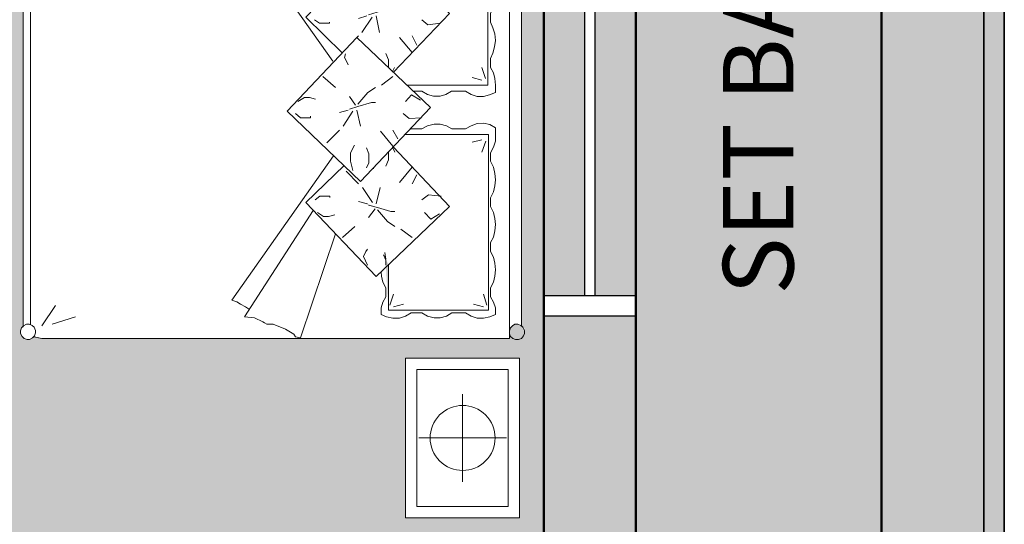
# Model space of a CAD drawing. Units: inches. Extents: x 528 to 2620, y -1066 to 798.
# Tile 14 of 41: x 848 to 944, y 573 to 623. Entities that reach past the tile are written whole.
import ezdxf

# ---------------------------------------------------------------- set-up
doc = ezdxf.new("R2010")
doc.units = ezdxf.units.IN
doc.header["$MEASUREMENT"] = 0
for name, color, linetype, lineweight in [('A-AREA-IDEN', 7, 'Continuous', 18), ('A-FURN', 30, 'Continuous', 18), ('A-GLAZ', 3, 'Continuous', 25), ('A-WALL', 7, 'Continuous', 50), ('A-WALL-PATT', 8, 'Continuous', 13), ('C-PROP', 5, 'Continuous', 35)]:
    doc.layers.add(name, color=color, linetype=linetype, lineweight=lineweight)
doc.styles.get("Standard").update_dxf_attribs({"font": 'arial.ttf'})

# ---------------------------------------------------------------- blocks, each defined once
blk = doc.blocks.new('d-bed-3')
at = {"color": 0, "linetype": 'ByBlock'}
for p, q in [((0, 0), (0, -0.5)), ((0.7, 0), (0, 0)), ((0.7, -0.5), (0.7, 0)), ((0.7817, -0.0054), (0.7857, 0.0078)), ((0.7817, -0.0054), (0.7857, 0.0078)), ((0.7857, 0.0078), (0.7968, 0.0166)), ((0.7857, 0.0078), (0.7968, 0.0166)), ((0.7968, 0.0166), (0.8078, 0.0211)), ((0.7968, 0.0166), (0.8078, 0.0211)), ((0.8078, 0.0211), (0.8209, 0.0211)), ((0.8078, 0.0211), (0.8209, 0.0211)), ((0.8209, 0.0211), (0.8349, 0.0144)), ((0.8209, 0.0211), (0.8349, 0.0144)), ((0.8349, 0.0144), (0.8409, 0.0078)), ((0.8349, 0.0144), (0.8429, 0.0056)), ((0.8389, 0.0078), (2.7305, 0.0078)), ((0.8409, 0.0078), (2.7305, 0.0078)), ((0.8429, 0.0056), (0.848, -0.0077)), ((2.7234, -0.0077), (2.7284, 0.0056)), ((2.7284, 0.0056), (2.7365, 0.0144)), ((2.7305, 0.0078), (2.7365, 0.0144)), ((2.7365, 0.0144), (2.7505, 0.0211)), ((2.7365, 0.0144), (2.7505, 0.0211)), ((2.7505, 0.0211), (2.7636, 0.0211)), ((2.7505, 0.0211), (2.7636, 0.0211)), ((2.7636, 0.0211), (2.7746, 0.0166)), ((2.7636, 0.0211), (2.7746, 0.0166)), ((2.7746, 0.0166), (2.7857, 0.0078)), ((2.7746, 0.0166), (2.7857, 0.0078)), ((2.7857, 0.0078), (2.7897, -0.0054)), ((2.7857, 0.0078), (2.7897, -0.0054)), ((2.8714, -0.5), (2.8714, 0)), ((2.8714, 0), (3.5714, 0)), ((3.5714, 0), (3.5714, -0.5)), ((0.7817, -0.0187), (0.7817, -0.0054)), ((0.7817, -0.0187), (0.7817, -0.0054)), ((0.7857, -0.0297), (0.7817, -0.0187)), ((0.7857, -0.0297), (0.7817, -0.0187)), ((0.7857, -2.0939), (0.7857, -0.0297)), ((0.7948, -0.0408), (0.7857, -0.0297)), ((0.7857, -0.032), (0.7857, -2.0939)), ((0.8058, -0.0452), (0.7948, -0.0408)), ((0.8319, -0.0408), (0.8188, -0.0452)), ((0.8409, -0.032), (0.8319, -0.0408)), ((0.848, -0.0209), (0.8409, -0.032)), ((0.848, -0.0077), (0.848, -0.0209)), ((2.7234, -0.0209), (2.7234, -0.0077)), ((2.7305, -0.032), (2.7234, -0.0209)), ((2.7395, -0.0408), (2.7305, -0.032)), ((2.7525, -0.0452), (2.7395, -0.0408)), ((2.7766, -0.0408), (2.7656, -0.0452)), ((2.7766, -0.0408), (2.7656, -0.0452)), ((2.7857, -0.0297), (2.7766, -0.0408)), ((2.7857, -0.0297), (2.7766, -0.0408)), ((2.7897, -0.0187), (2.7857, -0.0297)), ((2.7897, -0.0187), (2.7857, -0.0297)), ((2.7897, -0.0054), (2.7897, -0.0187)), ((2.7897, -0.0054), (2.7897, -0.0187)), ((0.05, -0.05), (0.05, -0.45)), ((0.65, -0.05), (0.05, -0.05)), ((0.35, -0.0576), (0.35, -0.4424)), ((0.65, -0.45), (0.65, -0.05)), ((0.8188, -0.0452), (0.8058, -0.0452)), ((2.7525, -0.0452), (0.8188, -0.0452)), ((2.7656, -0.0452), (2.7525, -0.0452)), ((2.7656, -0.0452), (2.7857, -0.0452)), ((2.7857, -0.0452), (2.7656, -0.0452)), ((2.7857, -2.0939), (2.7857, -0.0452)), ((2.9214, -0.45), (2.9214, -0.05)), ((2.9214, -0.05), (3.5214, -0.05)), ((3.2214, -0.0576), (3.2214, -0.4424)), ((3.5214, -0.05), (3.5214, -0.45)), ((0.8781, -0.1325), (0.8911, -0.1059)), ((0.8911, -0.1059), (0.9182, -0.1082)), ((0.9182, -0.1082), (0.9443, -0.1148)), ((0.9443, -0.1148), (0.9684, -0.128)), ((0.9684, -0.128), (1.0056, -0.128)), ((1.0056, -0.128), (1.0317, -0.117)), ((1.0317, -0.117), (1.0588, -0.1082)), ((1.0588, -0.1082), (1.0849, -0.1059)), ((1.0849, -0.1059), (1.113, -0.1104)), ((1.113, -0.1104), (1.1401, -0.117)), ((1.1401, -0.117), (1.1662, -0.128)), ((1.1662, -0.128), (1.2034, -0.128)), ((1.2034, -0.128), (1.2295, -0.117)), ((1.2295, -0.117), (1.2566, -0.1082)), ((1.2566, -0.1082), (1.2827, -0.1059)), ((1.2827, -0.1059), (1.3108, -0.1104)), ((1.3108, -0.1104), (1.3379, -0.117)), ((1.3379, -0.117), (1.362, -0.128)), ((1.362, -0.128), (1.4012, -0.128)), ((1.4012, -0.128), (1.4253, -0.117)), ((1.4253, -0.117), (1.4514, -0.1082)), ((1.4514, -0.1082), (1.4805, -0.1059)), ((1.4805, -0.1059), (1.5086, -0.1104)), ((1.5086, -0.1104), (1.5357, -0.117)), ((1.5357, -0.117), (1.5598, -0.128)), ((1.5598, -0.128), (1.5989, -0.128)), ((1.5989, -0.128), (1.623, -0.1148)), ((1.623, -0.1148), (1.6471, -0.1082)), ((1.6471, -0.1082), (1.6763, -0.1059)), ((1.6763, -0.1059), (1.7084, -0.1059)), ((1.7084, -0.1059), (1.7194, -0.1325)), ((1.8489, -0.1302), (1.863, -0.1059)), ((1.863, -0.1059), (1.8951, -0.1059)), ((1.8951, -0.1059), (1.9222, -0.1059)), ((1.9222, -0.1059), (1.9483, -0.1148)), ((1.9483, -0.1148), (1.9724, -0.128)), ((1.9724, -0.128), (2.0096, -0.128)), ((2.0096, -0.128), (2.0357, -0.1148)), ((2.0357, -0.1148), (2.0628, -0.1082)), ((2.0628, -0.1082), (2.0909, -0.1059)), ((2.0909, -0.1059), (2.117, -0.1082)), ((2.117, -0.1082), (2.1441, -0.1148)), ((2.1441, -0.1148), (2.1702, -0.128)), ((2.1702, -0.128), (2.2074, -0.128)), ((2.2074, -0.128), (2.2335, -0.1148)), ((2.2335, -0.1148), (2.2606, -0.1082)), ((2.2606, -0.1082), (2.2867, -0.1059)), ((2.2867, -0.1059), (2.3148, -0.1082)), ((2.3148, -0.1082), (2.3419, -0.1148)), ((2.3419, -0.1148), (2.366, -0.128)), ((2.366, -0.128), (2.4052, -0.128)), ((2.4052, -0.128), (2.4293, -0.1148)), ((2.4293, -0.1148), (2.4554, -0.1082)), ((2.4554, -0.1082), (2.4845, -0.1059)), ((2.4845, -0.1059), (2.5126, -0.1082)), ((2.5126, -0.1082), (2.5397, -0.1148)), ((2.5397, -0.1148), (2.5638, -0.128)), ((2.5638, -0.128), (2.6029, -0.128)), ((2.6029, -0.128), (2.627, -0.1148)), ((2.627, -0.1148), (2.6511, -0.1059)), ((2.6511, -0.1059), (2.6803, -0.1059)), ((2.6803, -0.1059), (2.6913, -0.1302)), ((0.8721, -0.159), (0.8781, -0.1325)), ((0.8741, -0.1866), (0.8721, -0.159)), ((0.9072, -0.5753), (0.9072, -0.1391)), ((0.9072, -0.1391), (1.6763, -0.1391)), ((0.9223, -0.1612), (0.9333, -0.2042)), ((0.9293, -0.1435), (0.9775, -0.1612)), ((1.6471, -0.1501), (1.5989, -0.1656)), ((1.6542, -0.1656), (1.6431, -0.2087)), ((1.6763, -0.1391), (1.6763, -0.4936)), ((1.7194, -0.1325), (1.7265, -0.159)), ((1.7265, -0.159), (1.7265, -0.1866)), ((1.8429, -0.159), (1.8489, -0.1302)), ((1.8449, -0.1866), (1.8429, -0.159)), ((2.6622, -0.1369), (1.8931, -0.1369)), ((1.8931, -0.1369), (1.8931, -0.5046)), ((1.9152, -0.1656), (1.9263, -0.2087)), ((1.9222, -0.1479), (1.9704, -0.1656)), ((2.6401, -0.1435), (2.5919, -0.159)), ((2.6471, -0.159), (2.6361, -0.202)), ((2.6622, -0.5753), (2.6622, -0.1369)), ((2.6913, -0.1302), (2.6973, -0.159)), ((2.6973, -0.159), (2.6973, -0.1866)), ((0.8831, -0.2131), (0.8741, -0.1866)), ((0.8962, -0.2374), (0.8831, -0.2131)), ((1.7174, -0.2131), (1.7024, -0.2374)), ((1.7265, -0.1866), (1.7174, -0.2131)), ((1.854, -0.2131), (1.8449, -0.1866)), ((1.867, -0.2374), (1.854, -0.2131)), ((2.6883, -0.2131), (2.6732, -0.2374)), ((2.6973, -0.1866), (2.6883, -0.2131)), ((0.1576, -0.25), (0.5424, -0.25)), ((0.8962, -0.2992), (0.8962, -0.2374)), ((1.7024, -0.2374), (1.7024, -0.2992)), ((1.867, -0.297), (1.867, -0.2374)), ((2.6732, -0.2374), (2.6732, -0.297)), ((3.4138, -0.25), (3.029, -0.25)), ((0.8831, -0.3235), (0.8962, -0.2992)), ((1.7024, -0.2992), (1.7174, -0.3235)), ((1.854, -0.3213), (1.867, -0.297)), ((2.6732, -0.297), (2.6883, -0.3213)), ((0.8761, -0.3489), (0.8831, -0.3235)), ((1.0538, -0.6294), (1.362, -0.3081)), ((1.362, -0.3081), (1.619, -0.5532)), ((1.7174, -0.3235), (1.7244, -0.3489)), ((1.8469, -0.3489), (1.854, -0.3213)), ((2.2074, -0.3081), (1.9483, -0.5532)), ((2.1632, -0.3445), (2.1572, -0.3997)), ((2.5146, -0.6294), (2.2074, -0.3081)), ((2.6883, -0.3213), (2.6953, -0.3489)), ((0.8761, -0.3776), (0.8761, -0.3489)), ((0.8831, -0.4041), (0.8761, -0.3776)), ((1.3289, -0.3511), (1.3068, -0.3909)), ((1.4052, -0.3467), (1.4122, -0.4019)), ((1.7244, -0.3776), (1.7174, -0.4041)), ((1.7244, -0.3489), (1.7244, -0.3776)), ((1.8469, -0.3754), (1.8469, -0.3489)), ((1.854, -0.4041), (1.8469, -0.3754)), ((2.2405, -0.3511), (2.2626, -0.3887)), ((2.6953, -0.3754), (2.6883, -0.4041)), ((2.6953, -0.3489), (2.6953, -0.3754)), ((0.8962, -0.4284), (0.8831, -0.4041)), ((0.8962, -0.4781), (0.8962, -0.4284)), ((1.3068, -0.3909), (1.3349, -0.4174)), ((1.4122, -0.4019), (1.3901, -0.4284)), ((1.4674, -0.7134), (1.7746, -0.3909)), ((1.7174, -0.4041), (1.7024, -0.4284)), ((1.7024, -0.4284), (1.7024, -0.4649)), ((1.7746, -0.3909), (2.0979, -0.6979)), ((1.8188, -0.4306), (1.8228, -0.4848)), ((1.867, -0.4284), (1.854, -0.4041)), ((1.867, -0.4781), (1.867, -0.4284)), ((2.1572, -0.3997), (2.1793, -0.4284)), ((2.2626, -0.3887), (2.2335, -0.4174)), ((2.6883, -0.4041), (2.6732, -0.4284)), ((2.6732, -0.4284), (2.6732, -0.4759)), ((0.05, -0.45), (0.65, -0.45)), ((1.2255, -0.4715), (1.2626, -0.5223)), ((1.5006, -0.4505), (1.4604, -0.4715)), ((1.5327, -0.4715), (1.4674, -0.5267)), ((1.7415, -0.4351), (1.7194, -0.4737)), ((1.7194, -0.4737), (1.7485, -0.5002)), ((2.0357, -0.4715), (2.102, -0.5267)), ((2.0688, -0.4505), (2.109, -0.4715)), ((2.3439, -0.4715), (2.3068, -0.5201)), ((3.5214, -0.45), (2.9214, -0.45)), ((0, -0.5), (0.7, -0.5)), ((0.8741, -0.5289), (0.8831, -0.5024)), ((0.8831, -0.5024), (0.8962, -0.4781)), ((0.9223, -0.5532), (0.9333, -0.5113)), ((1.8228, -0.4848), (1.8008, -0.5113)), ((2.6471, -0.5532), (2.6361, -0.5091)), ((2.6732, -0.4759), (2.6883, -0.5002)), ((2.6883, -0.5002), (2.6973, -0.5267)), ((3.5714, -0.5), (2.8714, -0.5)), ((0.8721, -0.5576), (0.8741, -0.5289)), ((0.8781, -0.5841), (0.8721, -0.5576)), ((0.9293, -0.5709), (0.9775, -0.5532)), ((1.2957, -0.5819), (1.2737, -0.5488)), ((1.3399, -0.5643), (1.3399, -0.5488)), ((1.5989, -0.5488), (1.614, -0.5554)), ((1.6381, -0.5554), (1.6763, -0.6051)), ((1.9112, -0.5333), (1.874, -0.5554)), ((1.9443, -0.5554), (1.8781, -0.6096)), ((1.9704, -0.5466), (1.9503, -0.5554)), ((2.2295, -0.5643), (2.2295, -0.5466)), ((2.2736, -0.5797), (2.2957, -0.5466)), ((2.6401, -0.5687), (2.5919, -0.5532)), ((2.6973, -0.5554), (2.6913, -0.5841)), ((2.6973, -0.5267), (2.6973, -0.5554)), ((0.8911, -0.6096), (0.8781, -0.5841)), ((1.109, -0.5753), (0.9072, -0.5753)), ((0.9443, -0.6007), (0.9182, -0.6073)), ((0.9684, -0.5886), (0.9443, -0.6007)), ((1.0056, -0.5886), (0.9684, -0.5886)), ((1.0317, -0.5996), (1.0056, -0.5886)), ((1.0588, -0.6073), (1.0317, -0.5996)), ((1.105, -0.5864), (1.1271, -0.5864)), ((1.1271, -0.5864), (1.1482, -0.5974)), ((1.1482, -0.5974), (1.1311, -0.5864)), ((1.1311, -0.5864), (1.1592, -0.593)), ((1.3459, -0.625), (1.2957, -0.5819)), ((1.357, -0.625), (1.3399, -0.5643)), ((1.5658, -0.5753), (1.5377, -0.5864)), ((1.5969, -0.5753), (1.5658, -0.5753)), ((1.9684, -0.5753), (2.0036, -0.5753)), ((2.0036, -0.5753), (2.0317, -0.5864)), ((2.2124, -0.6228), (2.2295, -0.5643)), ((2.2224, -0.6228), (2.2736, -0.5797)), ((2.4383, -0.5864), (2.4092, -0.5908)), ((2.4423, -0.5864), (2.4202, -0.5974)), ((2.4202, -0.5974), (2.4383, -0.5864)), ((2.4644, -0.5864), (2.4423, -0.5864)), ((2.4604, -0.5753), (2.6622, -0.5753)), ((2.5397, -0.5996), (2.5126, -0.6051)), ((2.5638, -0.5864), (2.5397, -0.5996)), ((2.6029, -0.5864), (2.5638, -0.5864)), ((2.627, -0.5996), (2.6029, -0.5864)), ((2.6511, -0.6073), (2.627, -0.5996)), ((2.6913, -0.5841), (2.6803, -0.6073)), ((0.9182, -0.6073), (0.8911, -0.6096)), ((1.3791, -0.9365), (1.0538, -0.6294)), ((1.0759, -0.6096), (1.0588, -0.6073)), ((1.3138, -0.6626), (1.351, -0.6361)), ((1.368, -0.6626), (1.357, -0.625)), ((1.3731, -0.6294), (1.4453, -0.614)), ((1.3791, -0.6471), (1.4453, -0.6913)), ((1.7084, -0.6648), (1.6873, -0.6316)), ((1.7526, -0.6493), (1.7526, -0.6316)), ((2.0387, -0.6427), (2.0427, -0.6405)), ((2.1963, -0.6294), (2.124, -0.6118)), ((2.1903, -0.6449), (2.124, -0.6891)), ((2.1903, -0.9365), (2.5146, -0.6294)), ((2.2013, -0.6626), (2.2124, -0.6228)), ((2.2556, -0.6626), (2.2184, -0.6338)), ((2.5126, -0.6051), (2.4955, -0.6073)), ((2.6803, -0.6073), (2.6511, -0.6073)), ((1.105, -0.6692), (1.1421, -0.6846)), ((1.1421, -0.6846), (1.1642, -0.6736)), ((1.1642, -0.6736), (1.1753, -0.6692)), ((1.3731, -0.6692), (1.3841, -0.7067)), ((1.7596, -0.7089), (1.7084, -0.6648)), ((1.7706, -0.7089), (1.7526, -0.6493)), ((1.9765, -0.6604), (1.9503, -0.6714)), ((2.0166, -0.6604), (1.9765, -0.6604)), ((2.0387, -0.6714), (2.0166, -0.6604)), ((2.1963, -0.667), (2.1853, -0.7067)), ((2.4052, -0.6736), (2.3941, -0.667)), ((2.4272, -0.6846), (2.4052, -0.6736)), ((2.4644, -0.667), (2.4272, -0.6846)), ((1.2255, -0.7785), (1.2737, -0.7244)), ((1.4674, -0.7134), (1.4604, -0.7067)), ((1.7897, -1.0193), (1.4674, -0.7134)), ((1.7265, -0.7454), (1.7636, -0.72)), ((1.7817, -0.7454), (1.7706, -0.7089)), ((1.7857, -0.7134), (1.856, -0.6979)), ((2.0979, -0.6979), (1.7897, -1.0193)), ((1.7897, -0.731), (1.856, -0.7741)), ((1.9724, -0.741), (1.9393, -0.7244)), ((2.0497, -0.731), (2.0096, -0.741)), ((2.0538, -0.7609), (2.109, -0.7067)), ((2.3439, -0.7763), (2.2957, -0.7222)), ((1.3791, -0.9365), (1.5357, -0.7763)), ((1.5548, -0.7675), (1.5397, -0.7631)), ((1.5548, -0.7675), (1.5769, -0.7564)), ((1.5769, -0.7564), (1.5879, -0.752)), ((1.7857, -0.752), (1.7967, -0.7896)), ((2.0096, -0.741), (1.9724, -0.741)), ((2.1903, -0.9365), (2.0277, -0.7697)), ((0.7857, -0.9607), (1.2295, -0.8072)), ((0.9504, -1.2611), (1.5708, -0.8183)), ((1.3178, -0.8382), (1.3239, -0.8117)), ((1.6381, -0.8625), (1.6873, -0.8072)), ((1.9283, -0.8448), (1.874, -0.7896)), ((2.618, -1.2611), (1.9855, -0.8161)), ((2.2515, -0.8382), (2.2445, -0.8094)), ((2.7827, -0.9607), (2.3278, -0.8072)), ((1.3178, -0.8602), (1.3178, -0.8382)), ((1.3349, -0.8879), (1.3178, -0.8602)), ((1.4052, -0.8337), (1.4012, -0.8337)), ((1.4052, -0.8768), (1.4052, -0.8337)), ((2.1632, -0.8757), (2.1632, -0.8315)), ((2.1632, -0.8315), (2.1682, -0.8315)), ((2.2335, -0.8856), (2.2515, -0.8602)), ((2.2515, -0.8602), (2.2515, -0.8382)), ((0.8781, -1.2059), (1.3349, -0.9055)), ((1.3901, -0.8989), (1.4052, -0.8768)), ((1.7305, -0.921), (1.7375, -0.8945)), ((2.1793, -0.8967), (2.1632, -0.8757)), ((2.6913, -1.2059), (2.2254, -0.9055)), ((1.7305, -0.9431), (1.7305, -0.921)), ((1.7485, -0.9718), (1.7305, -0.9431)), ((1.8188, -0.9166), (1.8118, -0.9166)), ((1.8188, -0.9607), (1.8188, -0.9166)), ((0.8128, -1.0115), (0.7857, -0.9607)), ((1.8008, -0.9828), (1.8188, -0.9607)), ((2.7676, -0.9895), (2.7455, -1.0259)), ((2.7786, -0.9828), (2.7676, -0.9895)), ((2.7827, -0.9607), (2.7786, -0.9828)), ((0.8128, -1.0325), (0.8128, -1.0115)), ((0.8239, -1.0414), (0.8128, -1.0325)), ((2.7455, -1.0259), (2.7234, -1.0811)), ((0.8299, -1.0635), (0.8239, -1.0414)), ((0.8349, -1.0745), (0.8299, -1.0635)), ((0.845, -1.1032), (0.8349, -1.0745)), ((0.852, -1.1187), (0.845, -1.1032)), ((0.852, -1.1363), (0.852, -1.1187)), ((2.7174, -1.1187), (2.7124, -1.1253)), ((2.7234, -1.1076), (2.7174, -1.1187)), ((2.7234, -1.0811), (2.7234, -1.1076)), ((0.863, -1.1617), (0.852, -1.1363)), ((0.867, -1.1905), (0.863, -1.1617)), ((2.6953, -1.1617), (2.6913, -1.2059)), ((2.7124, -1.1253), (2.6953, -1.1617)), ((0.8741, -1.1949), (0.867, -1.1905)), ((0.8781, -1.2059), (0.8741, -1.1949)), ((0.9223, -1.2015), (0.9112, -1.1838)), ((0.9293, -1.2059), (0.9223, -1.2015)), ((0.9403, -1.2236), (0.9293, -1.2059)), ((2.6471, -1.2015), (2.6361, -1.2236)), ((2.6582, -1.1838), (2.6471, -1.2015)), ((0.9443, -1.2391), (0.9403, -1.2236)), ((0.9504, -1.2611), (0.9443, -1.2391)), ((2.625, -1.2391), (2.618, -1.2611)), ((2.6361, -1.2236), (2.625, -1.2391)), ((0.8741, -2.0673), (0.9464, -1.9691)), ((2.7234, -2.0497), (2.6913, -1.947)), ((0.8851, -2.1005), (0.9795, -2.0342)), ((2.7305, -2.0939), (2.6421, -2.0342)), ((0.7888, -2.1317), (0.7857, -2.0939)), ((0.7857, -2.0939), (0.7887, -2.1303)), ((2.7857, -2.0939), (2.7783, -2.1299)), ((2.7786, -2.1281), (2.7857, -2.0939)), ((0.7797, -2.148), (0.7857, -2.1347)), ((0.7797, -2.148), (0.7857, -2.1347)), ((0.7797, -2.159), (0.7797, -2.148)), ((0.7797, -2.148), (0.7797, -2.159)), ((0.7857, -2.1347), (0.7948, -2.1259)), ((0.7857, -2.1347), (0.7888, -2.1317)), ((0.7948, -2.1259), (0.8078, -2.1215)), ((0.8078, -2.1215), (0.8188, -2.1215)), ((0.8188, -2.1215), (0.8319, -2.1281)), ((0.8319, -2.1281), (0.8409, -2.1369)), ((0.8409, -2.1369), (0.845, -2.1502)), ((2.7264, -2.1436), (0.845, -2.1436)), ((0.845, -2.1502), (0.845, -2.1612)), ((2.7284, -2.1369), (2.7234, -2.1502)), ((2.7234, -2.1502), (2.7234, -2.1612)), ((2.7365, -2.1281), (2.7284, -2.1369)), ((2.7505, -2.1215), (2.7365, -2.1281)), ((2.7616, -2.1215), (2.7505, -2.1215)), ((2.7746, -2.1259), (2.7616, -2.1215)), ((2.7827, -2.1347), (2.7746, -2.1259)), ((2.7783, -2.1299), (2.7827, -2.1347)), ((2.7827, -2.1347), (2.7897, -2.148)), ((2.7897, -2.148), (2.7827, -2.1347)), ((2.7897, -2.148), (2.7897, -2.159)), ((2.7897, -2.159), (2.7897, -2.148)), ((0.7837, -2.1723), (0.7797, -2.159)), ((0.7837, -2.1723), (0.7797, -2.159)), ((0.7927, -2.1811), (0.7837, -2.1723)), ((0.7927, -2.1811), (0.7837, -2.1723)), ((0.8058, -2.1877), (0.7927, -2.1811)), ((0.8058, -2.1877), (0.7927, -2.1811)), ((0.8168, -2.1877), (0.8058, -2.1877)), ((0.8168, -2.1877), (0.8058, -2.1877)), ((0.8299, -2.1833), (0.8168, -2.1877)), ((0.8299, -2.1833), (0.8168, -2.1877)), ((0.8389, -2.1745), (0.8299, -2.1833)), ((0.8367, -2.1767), (0.8299, -2.1833)), ((2.7327, -2.1767), (0.8367, -2.1767)), ((0.845, -2.1612), (0.8389, -2.1745)), ((0.8389, -2.1767), (2.7305, -2.1767)), ((2.7234, -2.1612), (2.7305, -2.1745)), ((2.7305, -2.1745), (2.7395, -2.1833)), ((2.7395, -2.1833), (2.7327, -2.1767)), ((2.7525, -2.1877), (2.7395, -2.1833)), ((2.7395, -2.1833), (2.7525, -2.1877)), ((2.7636, -2.1877), (2.7525, -2.1877)), ((2.7525, -2.1877), (2.7636, -2.1877)), ((2.7766, -2.1811), (2.7636, -2.1877)), ((2.7636, -2.1877), (2.7766, -2.1811)), ((2.7857, -2.1723), (2.7766, -2.1811)), ((2.7766, -2.1811), (2.7857, -2.1723)), ((2.7897, -2.159), (2.7857, -2.1723)), ((2.7857, -2.1723), (2.7897, -2.159))]:
    blk.add_line(p, q, dxfattribs=at)
blk.add_ellipse((0.35, -0.25), major_axis=(-0.1007, 0.1007), ratio=1, dxfattribs=at)
at = {"color": 0, "linetype": 'ByBlock', "extrusion": (0, 0, -1)}
blk.add_ellipse((3.2214, -0.25), major_axis=(0.1007, 0.1007), ratio=1, dxfattribs=at)
blk = doc.blocks.new('WIN-1200')
for p, q in [((677.559, 718.922), (725.559, 718.922)), ((677.559, 709.922), (677.559, 718.922)), ((679.559, 709.922), (679.559, 718.922)), ((723.559, 718.922), (723.559, 709.922)), ((725.559, 718.922), (725.559, 709.922)), ((679.559, 714.922), (723.559, 714.922)), ((679.559, 713.922), (723.559, 713.922)), ((725.559, 709.922), (677.559, 709.922))]:
    blk.add_line(p, q)

msp = doc.modelspace()

# ---------------------------------------------------------------- hatches: boundary and pattern name
at = {"layer": 'A-WALL-PATT', "transparency": 33554687}
h = msp.add_hatch(color=256, dxfattribs=at)
h.dxf.hatch_style = 1
h.paths.add_polyline_path([(944.059, 753.922), (584.059, 753.922), (584.059, 208.922), (608.059, 208.922), (608.059, 210.922), (586.059, 210.922), (586.059, 751.922), (942.059, 751.922), (942.059, 210.922), (728.059, 210.922), (728.059, 208.922), (944.059, 208.922)])
h = msp.add_hatch(color=256, dxfattribs=at)
h.dxf.hatch_style = 1
h.paths.add_polyline_path([(942.059, 751.922), (586.059, 751.922), (586.059, 210.922), (608.059, 210.922), (608.059, 220.922), (596.059, 220.922), (596.059, 741.922), (932.059, 741.922), (932.059, 220.922), (770.059, 220.922), (728.059, 220.922), (728.059, 210.922), (942.059, 210.922)])
at = {"layer": 'A-WALL-PATT', "transparency": 33554475}
h = msp.add_hatch(color=256, dxfattribs=at)
h.dxf.hatch_style = 1
h.paths.add_polyline_path([(620.059, 718.922), (908.059, 718.922), (908.059, 268.922), (770.059, 268.922), (770.059, 220.922), (932.059, 220.922), (932.059, 741.922), (596.059, 741.922), (596.059, 391.422), (620.059, 391.422)])
at = {"layer": 'A-WALL-PATT', "transparency": 33554687}
h = msp.add_hatch(color=256, dxfattribs=at)
h.dxf.hatch_style = 1
h.paths.add_polyline_path([(861.059, 273.922), (817.059, 273.922), (817.059, 272.922), (861.059, 272.922)])
h.paths.add_polyline_path([(817.059, 277.922), (815.059, 277.922), (815.059, 268.922), (817.059, 268.922)])
h.paths.add_polyline_path([(908.059, 397.922), (899.059, 397.922), (899.059, 395.922), (908.059, 395.922)])
h.paths.add_polyline_path([(908.059, 443.922), (899.059, 443.922), (899.059, 441.922), (908.059, 441.922)])
h.paths.add_polyline_path([(904.059, 441.922), (903.059, 441.922), (903.059, 397.922), (904.059, 397.922)])
h.paths.add_polyline_path([(625.059, 561.422), (624.059, 561.422), (624.059, 537.422), (625.059, 537.422)])
h.paths.add_polyline_path([(648.747, 334.444), (720.045, 334.444), (720.045, 344.998), (648.747, 344.998)], flags=9)
h.paths.add_polyline_path([(819.733, 323.153), (880.328, 323.153), (880.328, 333.708), (819.733, 333.708)], flags=9)
h.paths.add_polyline_path([(779.898, 680.607), (821.764, 680.607), (821.764, 691.169), (779.898, 691.169)], flags=9)
h.paths.add_polyline_path([(779.876, 692.362), (817.138, 692.362), (817.138, 703.058), (779.876, 703.058)], flags=9)
h.paths.add_polyline_path([(799.994, 453.884), (860.589, 453.884), (860.589, 464.439), (799.994, 464.439)], flags=9)
h.paths.add_polyline_path([(650.866, 539.397), (708.781, 539.397), (708.781, 549.952), (650.866, 549.952)], flags=9)
h.paths.add_polyline_path([(788.504, 612.01), (849.099, 612.01), (849.099, 622.565), (788.504, 622.565)], flags=9)
h.paths.add_polyline_path([(639.539, 648.31), (700.134, 648.31), (700.134, 658.865), (639.539, 658.865)], flags=9)
h.paths.add_polyline_path([(648.913, 346.09), (747.706, 346.09), (747.706, 356.778), (648.913, 356.778)], flags=9)
h.paths.add_polyline_path([(676.857, 450.66), (746.735, 450.66), (746.735, 461.355), (676.857, 461.355)], flags=9)
h.paths.add_polyline_path([(819.711, 334.947), (865.526, 334.947), (865.526, 345.636), (819.711, 345.636)], flags=9)
h.paths.add_polyline_path([(806.298, 467.745), (874.047, 467.745), (874.047, 478.441), (806.298, 478.441)], flags=9)
h.paths.add_polyline_path([(653.235, 552.284), (690.497, 552.284), (690.497, 562.979), (653.235, 562.979)], flags=9)
h.paths.add_polyline_path([(789.903, 623.407), (843.208, 623.407), (843.208, 634.103), (789.903, 634.103)], flags=9)
h.paths.add_polyline_path([(639.773, 662.103), (693.077, 662.103), (693.077, 672.798), (639.773, 672.798)], flags=9)
h.paths.add_polyline_path([(801.587, 242.914), (846.334, 242.914), (846.334, 253.603), (801.587, 253.603)], flags=9)
h.paths.add_polyline_path([(925.362, 593.982), (925.362, 674.057), (914.673, 674.057), (914.673, 593.982)], flags=9)
h.paths.add_polyline_path([(612.559, 593.982), (612.559, 674.057), (601.871, 674.057), (601.871, 593.982)], flags=9)
h.paths.add_polyline_path([(723.31, 726.564), (803.385, 726.564), (803.385, 737.252), (723.31, 737.252)], flags=9)
at = {"layer": 'A-WALL-PATT', "transparency": 33554521}
h = msp.add_hatch(color=256, dxfattribs=at)
h.dxf.hatch_style = 1
h.paths.add_polyline_path([(629.059, 709.922), (677.559, 709.922), (677.559, 718.922), (620.059, 718.922), (620.059, 667.922), (629.059, 667.922)])
h.paths.add_polyline_path([(790.559, 718.922), (725.559, 718.922), (725.559, 709.922), (774.059, 709.922), (774.059, 577.922), (768.481, 577.922), (768.559, 573.422), (774.059, 573.422), (774.059, 567.422), (778.559, 567.422), (778.559, 669.422), (831.059, 669.422), (831.059, 675.922), (826.559, 675.922), (826.559, 673.922), (778.559, 673.922), (778.559, 709.922), (790.559, 709.922)])
h.paths.add_polyline_path([(908.059, 718.922), (879.059, 718.922), (879.059, 709.922), (899.059, 709.922), (899.059, 641.672), (908.059, 641.672)])
h.paths.add_polyline_path([(629.059, 619.922), (620.059, 619.922), (620.059, 561.422), (629.059, 561.422), (629.059, 573.422), (724.059, 573.422), (724.059, 569.422), (728.559, 569.422), (728.559, 577.922), (629.059, 577.922)])
h.paths.add_polyline_path([(779.059, 391.422), (779.059, 400.422), (770.059, 400.422), (764.059, 400.422), (764.059, 397.422), (764.059, 391.422), (770.059, 391.422), (770.059, 268.922), (815.059, 268.922), (815.059, 277.922), (779.059, 277.922), (779.059, 359.767)])
h.paths.add_polyline_path([(908.059, 395.922), (899.059, 395.922), (851.059, 395.922), (851.059, 391.422), (899.059, 391.422), (899.059, 277.922), (863.059, 277.922), (863.059, 268.922), (908.059, 268.922)])
h.paths.add_polyline_path([(908.059, 593.672), (899.059, 593.672), (899.059, 525.422), (778.559, 525.422), (778.559, 527.172), (774.059, 527.172), (774.059, 520.922), (899.059, 520.922), (899.059, 443.922), (908.059, 443.922)])
h.paths.add_polyline_path([(629.059, 520.922), (728.559, 520.922), (728.559, 545.422), (724.059, 545.422), (724.059, 525.422), (629.059, 525.422), (629.059, 537.422), (620.059, 537.422), (620.059, 484.672), (629.059, 484.672)])
h.paths.add_polyline_path([(629.059, 436.672), (620.059, 436.672), (620.059, 391.422), (648.559, 391.422), (648.559, 400.422), (629.059, 400.422)])
h.paths.add_polyline_path([(716.059, 397.422), (716.059, 400.422), (696.559, 400.422), (696.559, 391.422), (716.059, 391.422)])
at = {"layer": 'A-WALL-PATT', "transparency": 33554681}
h = msp.add_hatch(color=256, dxfattribs=at)
h.dxf.hatch_style = 1
h.paths.add_polyline_path([(629.059, 665.922), (625.059, 665.922), (625.059, 621.922), (629.059, 621.922)])
h.paths.add_polyline_path([(624.059, 665.922), (620.059, 665.922), (620.059, 621.922), (624.059, 621.922)])
h.paths.add_polyline_path([(723.559, 713.922), (679.559, 713.922), (679.559, 709.922), (723.559, 709.922)])
h.paths.add_polyline_path([(723.559, 718.922), (679.559, 718.922), (679.559, 714.922), (723.559, 714.922)])
h.paths.add_polyline_path([(814.559, 713.922), (790.559, 713.922), (790.559, 709.922), (814.559, 709.922)])
h.paths.add_polyline_path([(814.559, 718.922), (790.559, 718.922), (790.559, 714.922), (814.559, 714.922)])
h.paths.add_polyline_path([(877.059, 713.922), (833.059, 713.922), (833.059, 709.922), (877.059, 709.922)])
h.paths.add_polyline_path([(877.059, 718.922), (833.059, 718.922), (833.059, 714.922), (877.059, 714.922)])
h.paths.add_polyline_path([(908.059, 639.672), (904.059, 639.672), (904.059, 595.672), (908.059, 595.672)])
h.paths.add_polyline_path([(903.059, 639.672), (899.059, 639.672), (899.059, 595.672), (903.059, 595.672)])
h.paths.add_polyline_path([(908.059, 441.922), (904.059, 441.922), (904.059, 397.922), (908.059, 397.922)])
h.paths.add_polyline_path([(903.059, 441.922), (899.059, 441.922), (899.059, 397.922), (903.059, 397.922)])
h.paths.add_polyline_path([(861.059, 272.922), (817.059, 272.922), (817.059, 268.922), (861.059, 268.922)])
h.paths.add_polyline_path([(861.059, 277.922), (817.059, 277.922), (817.059, 273.922), (861.059, 273.922)])
h.paths.add_polyline_path([(694.559, 395.422), (650.559, 395.422), (650.559, 391.422), (694.559, 391.422)])
h.paths.add_polyline_path([(694.559, 400.422), (650.559, 400.422), (650.559, 396.422), (694.559, 396.422)])
h.paths.add_polyline_path([(629.059, 482.672), (625.059, 482.672), (625.059, 438.672), (629.059, 438.672)])
h.paths.add_polyline_path([(624.059, 482.672), (620.059, 482.672), (620.059, 438.672), (624.059, 438.672)])
h.paths.add_polyline_path([(629.059, 561.422), (625.059, 561.422), (625.059, 537.422), (629.059, 537.422)])
h.paths.add_polyline_path([(624.059, 561.422), (620.059, 561.422), (620.059, 537.422), (624.059, 537.422)])
at = {"layer": 'A-WALL-PATT', "transparency": 33554590}
h = msp.add_hatch(color=256, dxfattribs=at)
h.dxf.hatch_style = 1
h.paths.add_polyline_path([(774.059, 709.922), (629.059, 709.922), (629.059, 577.922), (728.559, 577.922), (728.559, 579.422), (728.559, 619.422), (730.309, 619.422), (730.309, 619.384, -0.401453), (768.559, 579.422), (768.559, 577.922), (774.059, 577.922)])
h.paths.add_polyline_path([(723.896, 686.058), (723.968, 686.064), (723.828, 686.128)], flags=0)
h.paths.add_polyline_path([(722.785, 642.699), (722.893, 642.756), (722.893, 684.992), (722.647, 685.244), (722.647, 685.82), (723.079, 686.262), (723.533, 686.262), (723.968, 686.064), (724.739, 686.128), (770.696, 686.128), (770.78, 686.14), (771.126, 686.266), (771.694, 686.094), (771.94, 685.478), (771.67, 684.904), (771.582, 684.871), (771.582, 642.782), (771.878, 642.514), (771.878, 641.921), (771.511, 641.462), (770.855, 641.462), (770.401, 641.833), (770.401, 641.551), (724.739, 641.551), (723.991, 641.705), (723.443, 641.414), (722.879, 641.585), (722.597, 642.142)], flags=16)
h.paths.add_polyline_path([(723.994, 641.704), (723.994, 641.707), (723.991, 641.705)], flags=0)
h.paths.add_polyline_path([(722.893, 642.732), (722.893, 684.992), (722.647, 685.244), (722.647, 685.82), (723.079, 686.262), (723.287, 686.262), (722.991, 686.172), (722.794, 685.971), (722.647, 685.68), (722.647, 685.434), (722.745, 685.143), (722.942, 684.942), (723.238, 684.807), (723.484, 684.807), (723.779, 684.897), (723.976, 685.098), (724.174, 685.488), (724.124, 685.635), (724.124, 685.249), (723.631, 684.746), (723.631, 642.961), (724.124, 642.514), (724.124, 641.887), (723.656, 641.462), (723.079, 641.462), (722.647, 641.904), (722.647, 642.48)], flags=0)
h.paths.add_polyline_path([(722.647, 642.29), (722.647, 642.044), (722.794, 641.753), (723.079, 641.462), (723.287, 641.462), (722.879, 641.585), (722.597, 642.142)], flags=0)
h.paths.add_polyline_path([(770.745, 686.128), (770.58, 686.128), (770.551, 686.057)], flags=0)
h.paths.add_polyline_path([(743.299, 645.288), (753.227, 659.398), (748.69, 663.75), (753.234, 668.538), (743.299, 682.458), (743.791, 682.592), (744.136, 682.681), (744.53, 682.928), (744.628, 683.084), (745.017, 683.327), (744.53, 684.069), (744.776, 684.158), (744.874, 684.315), (745.514, 684.404), (746.081, 684.651), (746.474, 684.651), (746.819, 684.807), (747.459, 685.031), (747.705, 685.143), (748.198, 685.277), (748.394, 685.523), (748.862, 685.523), (749.994, 686.128), (753.488, 676.03), (757.379, 680.153), (757.791, 679.758), (758.044, 680.645), (758.29, 681.227), (758.29, 682.055), (758.019, 682.592), (757.871, 683.174), (757.822, 683.778), (758.388, 684.069), (758.979, 684.203), (759.619, 684.158), (760.21, 683.957), (760.751, 683.666), (761.859, 683.666), (762.401, 683.957), (762.991, 684.114), (763.631, 684.114), (764.198, 683.957), (764.739, 683.666), (766.118, 683.666), (766.659, 683.957), (767.25, 684.158), (767.865, 684.203), (768.456, 684.069), (769.047, 683.778), (768.998, 683.174), (768.85, 682.592), (768.554, 682.055), (768.554, 681.227), (768.801, 680.645), (769.092, 679.75), (768.948, 678.832), (768.801, 678.228), (768.554, 677.646), (768.554, 676.818), (768.801, 676.237), (769.092, 675.341), (768.948, 674.424), (768.801, 673.82), (768.554, 673.283), (768.554, 672.41), (768.801, 671.873), (768.998, 671.291), (769.047, 670.642), (768.948, 670.016), (768.801, 669.411), (768.554, 668.874), (768.554, 668.002), (768.974, 667.239), (769.047, 666.279), (769.047, 665.563), (768.456, 665.316), (767.865, 665.16), (767.25, 665.16), (766.659, 665.361), (766.118, 665.697), (764.739, 665.697), (763.945, 665.204), (762.991, 665.204), (762.401, 665.361), (761.859, 665.697), (761.005, 665.697), (762.696, 664.086), (760.741, 662.027), (761.859, 662.027), (762.401, 662.318), (763.342, 662.548), (764.247, 662.318), (764.788, 662.027), (766.118, 662.027), (766.659, 662.318), (767.25, 662.519), (767.865, 662.564), (768.505, 662.43), (769.047, 662.116), (769.047, 661.4), (769.047, 660.796), (768.85, 660.214), (768.554, 659.677), (768.554, 658.849), (768.85, 658.267), (768.998, 657.663), (769.069, 656.749), (768.85, 655.851), (768.554, 655.269), (768.554, 654.441), (768.85, 653.859), (769.069, 652.961), (768.998, 652.046), (768.85, 651.442), (768.554, 650.905), (768.554, 650.032), (768.85, 649.495), (768.998, 648.914), (769.047, 648.265), (768.998, 647.638), (768.85, 647.034), (768.554, 646.497), (768.554, 645.624), (768.85, 645.087), (769.047, 644.55), (769.047, 643.901), (768.505, 643.655), (767.865, 643.521), (767.25, 643.521), (766.659, 643.722), (766.118, 644.058), (764.788, 644.058), (764.247, 643.722), (763.342, 643.492), (762.401, 643.722), (761.859, 644.058), (760.801, 644.058), (760.259, 643.722), (759.668, 643.521), (759.028, 643.521), (758.388, 643.655), (757.871, 643.901), (757.871, 644.55), (758.044, 645.087), (758.339, 645.624), (758.339, 646.497), (758.044, 647.034), (757.921, 647.638), (757.866, 648.059), (757.379, 647.593), (753.422, 651.773), (749.994, 641.618), (749.502, 641.708), (749.354, 641.954), (748.542, 642.446), (747.311, 642.939), (746.652, 642.939), (746.327, 643.185), (745.514, 643.565), (744.53, 643.655), (745.011, 644.4), (744.628, 644.639), (744.136, 644.886), (743.791, 645.132)], flags=0)
h.paths.add_polyline_path([(755.656, 654.933), (756.542, 654.687), (757.527, 654.329), (756.641, 654.575)], flags=0)
h.paths.add_polyline_path([(758.339, 649.204), (758.339, 648.712), (758.585, 644.304), (758.585, 648.802)], flags=0)
h.paths.add_polyline_path([(758.339, 649.294), (758.093, 649.697), (758.359, 649.165)], flags=0)
h.paths.add_polyline_path([(755.656, 672.79), (756.493, 673.037), (757.358, 673.351), (757.353, 673.358), (756.641, 673.149)], flags=0)
h.paths.add_polyline_path([(760.264, 639.641), (771.408, 639.641), (771.408, 624.039), (760.264, 624.039)], flags=16)
h.paths.add_polyline_path([(761.378, 638.526), (770.294, 638.526), (770.294, 625.153), (761.378, 625.153)], flags=0)
edge = h.paths.add_edge_path(flags=0)
edge.add_ellipse((765.836, 631.84), major_axis=(-2.245, 2.245), ratio=1, start_angle=-45, end_angle=45, ccw=False)
edge.add_ellipse((765.836, 631.84), major_axis=(-2.245, 2.245), ratio=1, start_angle=-135, end_angle=-45, ccw=False)
edge.add_ellipse((765.836, 631.84), major_axis=(-2.245, 2.245), ratio=1, start_angle=135, end_angle=-135, ccw=False)
edge.add_ellipse((765.836, 631.84), major_axis=(-2.245, 2.245), ratio=1, start_angle=45, end_angle=135, ccw=False)
h.paths.add_polyline_path([(758.585, 683.42), (758.585, 678.922), (758.373, 678.575), (758.339, 678.43), (758.093, 678.049), (758.339, 678.519), (758.339, 679.011)], flags=0)
h.paths.add_polyline_path([(760.264, 688.038), (760.264, 703.64), (771.408, 703.64), (771.408, 688.038)], flags=16)
h.paths.add_polyline_path([(770.401, 685.389), (770.401, 685.846), (770.855, 686.217), (771.511, 686.217), (771.878, 685.758), (771.878, 685.165), (771.582, 684.897), (771.582, 642.782), (771.878, 642.514), (771.878, 641.921), (771.511, 641.462), (770.855, 641.462), (770.401, 641.833), (770.401, 642.29)], flags=0)
h.paths.add_polyline_path([(770.532, 642.678), (771.052, 643.009), (771.67, 642.775), (771.94, 642.201), (771.694, 641.585), (771.126, 641.413), (770.551, 641.622), (770.347, 642.132)], flags=16)
h.paths.add_polyline_path([(761.378, 689.152), (761.378, 702.526), (770.294, 702.526), (770.294, 689.152)], flags=0)
edge = h.paths.add_edge_path(flags=0)
edge.add_ellipse((765.836, 695.839), major_axis=(2.245, 2.245), ratio=1, start_angle=405, end_angle=495, ccw=False)
edge.add_ellipse((765.836, 695.839), major_axis=(2.245, 2.245), ratio=1, start_angle=675, end_angle=765, ccw=False)
edge.add_ellipse((765.836, 695.839), major_axis=(2.245, 2.245), ratio=1, start_angle=585, end_angle=675, ccw=False)
edge.add_ellipse((765.836, 695.839), major_axis=(2.245, 2.245), ratio=1, start_angle=495, end_angle=585, ccw=False)
h.paths.add_polyline_path([(770.696, 684.897), (770.942, 684.74), (771.41, 684.74), (771.73, 685.031), (771.878, 685.344), (771.878, 685.635), (771.694, 686.094), (771.582, 686.128), (771.878, 685.758), (771.878, 685.165), (771.41, 684.74), (770.849, 684.74)], flags=0)
h.paths.add_polyline_path([(899.059, 709.922), (831.059, 709.922), (831.059, 699.922), (829.809, 699.922), (829.809, 675.922), (831.059, 675.922), (831.059, 669.422), (778.559, 669.422), (778.559, 567.172), (780.059, 567.172), (820.059, 567.172), (820.059, 565.422), (820.021, 565.422, -0.401453), (780.059, 527.172), (778.559, 527.172), (778.559, 525.422), (899.059, 525.422)])
h.paths.add_polyline_path([(849.197, 636.014), (849.269, 636.02), (849.129, 636.084)], flags=0)
h.paths.add_polyline_path([(848.193, 634.948), (847.947, 635.2), (847.947, 635.776), (848.379, 636.218), (848.833, 636.218), (849.269, 636.02), (850.039, 636.084), (895.996, 636.084), (896.081, 636.096), (896.426, 636.222), (896.995, 636.05), (897.241, 635.434), (896.97, 634.86), (896.883, 634.827), (896.883, 592.738), (897.178, 592.47), (897.178, 591.877), (896.811, 591.418), (896.155, 591.418), (895.701, 591.789), (895.701, 591.507), (850.039, 591.507), (849.292, 591.661), (848.744, 591.37), (848.18, 591.541), (847.897, 592.098), (848.086, 592.655), (848.193, 592.712)], flags=16)
h.paths.add_polyline_path([(849.294, 591.66), (849.295, 591.663), (849.292, 591.661)], flags=16)
h.paths.add_polyline_path([(848.193, 634.948), (847.947, 635.2), (847.947, 635.776), (848.379, 636.218), (848.587, 636.218), (848.292, 636.128), (848.095, 635.927), (847.947, 635.636), (847.947, 635.39), (848.046, 635.099), (848.243, 634.897), (848.538, 634.763), (848.784, 634.763), (849.079, 634.853), (849.276, 635.054), (849.474, 635.444), (849.424, 635.591), (849.424, 635.205), (848.932, 634.702), (848.932, 592.917), (849.424, 592.47), (849.424, 591.843), (848.956, 591.418), (848.379, 591.418), (847.947, 591.86), (847.947, 592.436), (848.193, 592.688)], flags=0)
h.paths.add_polyline_path([(847.947, 592.246), (847.947, 592), (848.095, 591.709), (848.379, 591.418), (848.587, 591.418), (848.18, 591.541), (847.897, 592.098)], flags=16)
h.paths.add_polyline_path([(896.046, 636.084), (895.88, 636.084), (895.852, 636.013)], flags=0)
h.paths.add_polyline_path([(868.599, 632.414), (869.092, 632.548), (869.436, 632.637), (869.83, 632.884), (869.929, 633.04), (870.318, 633.283), (869.83, 634.025), (870.076, 634.114), (870.175, 634.271), (870.815, 634.36), (871.381, 634.607), (871.775, 634.607), (872.119, 634.763), (872.759, 634.987), (873.006, 635.099), (873.498, 635.233), (873.695, 635.479), (874.163, 635.479), (875.295, 636.084), (878.788, 625.986), (882.679, 630.109), (883.091, 629.714), (883.344, 630.601), (883.59, 631.183), (883.59, 632.011), (883.319, 632.548), (883.172, 633.13), (883.123, 633.734), (883.689, 634.025), (884.279, 634.159), (884.919, 634.114), (885.51, 633.913), (886.052, 633.622), (887.159, 633.622), (887.701, 633.913), (888.292, 634.07), (888.932, 634.07), (889.498, 633.913), (890.039, 633.622), (891.418, 633.622), (891.959, 633.913), (892.55, 634.114), (893.166, 634.159), (893.756, 634.025), (894.347, 633.734), (894.298, 633.13), (894.15, 632.548), (893.855, 632.011), (893.855, 631.183), (894.101, 630.601), (894.393, 629.706), (894.249, 628.788), (894.101, 628.184), (893.855, 627.602), (893.855, 626.774), (894.101, 626.193), (894.393, 625.297), (894.249, 624.38), (894.101, 623.776), (893.855, 623.239), (893.855, 622.366), (894.101, 621.829), (894.298, 621.247), (894.347, 620.598), (894.249, 619.972), (894.101, 619.367), (893.855, 618.83), (893.855, 617.958), (894.274, 617.195), (894.347, 616.235), (894.347, 615.518), (893.756, 615.272), (893.166, 615.116), (892.55, 615.116), (891.959, 615.317), (891.418, 615.653), (890.039, 615.653), (889.245, 615.16), (888.292, 615.16), (887.701, 615.317), (887.159, 615.653), (886.305, 615.653), (887.996, 614.042), (886.041, 611.983), (887.159, 611.983), (887.701, 612.274), (888.642, 612.504), (889.547, 612.274), (890.089, 611.983), (891.418, 611.983), (891.959, 612.274), (892.55, 612.475), (893.166, 612.52), (893.806, 612.386), (894.347, 612.072), (894.347, 611.356), (894.347, 610.752), (894.15, 610.17), (893.855, 609.633), (893.855, 608.805), (894.15, 608.223), (894.298, 607.619), (894.37, 606.705), (894.15, 605.807), (893.855, 605.225), (893.855, 604.397), (894.15, 603.815), (894.37, 602.917), (894.298, 602.002), (894.15, 601.398), (893.855, 600.861), (893.855, 599.988), (894.15, 599.451), (894.298, 598.87), (894.347, 598.221), (894.298, 597.594), (894.15, 596.99), (893.855, 596.453), (893.855, 595.58), (894.15, 595.043), (894.347, 594.506), (894.347, 593.857), (893.806, 593.611), (893.166, 593.477), (892.55, 593.477), (891.959, 593.678), (891.418, 594.014), (890.089, 594.014), (889.547, 593.678), (888.642, 593.448), (887.701, 593.678), (887.159, 594.014), (886.101, 594.014), (885.559, 593.678), (884.969, 593.477), (884.329, 593.477), (883.689, 593.611), (883.172, 593.857), (883.172, 594.506), (883.344, 595.043), (883.639, 595.58), (883.639, 596.453), (883.344, 596.99), (883.221, 597.594), (883.167, 598.015), (882.679, 597.549), (878.722, 601.729), (875.295, 591.574), (874.803, 591.664), (874.655, 591.91), (873.843, 592.402), (872.612, 592.895), (871.952, 592.895), (871.627, 593.141), (870.815, 593.521), (869.83, 593.611), (870.311, 594.356), (869.929, 594.595), (869.436, 594.842), (869.092, 595.088), (868.599, 595.244), (878.528, 609.354), (873.99, 613.706), (878.535, 618.494)], flags=0)
h.paths.add_polyline_path([(880.956, 622.746), (881.793, 622.993), (882.659, 623.307), (882.654, 623.314), (881.941, 623.104)], flags=0)
h.paths.add_polyline_path([(880.956, 604.889), (881.843, 604.643), (882.827, 604.285), (881.941, 604.531)], flags=16)
h.paths.add_polyline_path([(883.393, 628.005), (883.639, 628.475), (883.639, 628.967), (883.886, 633.376), (883.886, 628.878), (883.674, 628.531), (883.639, 628.386)], flags=0)
h.paths.add_polyline_path([(883.639, 599.16), (883.639, 598.668), (883.886, 594.26), (883.886, 598.758)], flags=16)
h.paths.add_polyline_path([(883.639, 599.25), (883.393, 599.653), (883.659, 599.121)], flags=16)
h.paths.add_polyline_path([(885.564, 637.994), (885.564, 653.596), (896.709, 653.596), (896.709, 637.994)], flags=16)
h.paths.add_polyline_path([(885.564, 589.597), (896.709, 589.597), (896.709, 573.995), (885.564, 573.995)], flags=16)
h.paths.add_polyline_path([(886.679, 639.108), (886.679, 652.482), (895.594, 652.482), (895.594, 639.108)], flags=0)
h.paths.add_polyline_path([(886.679, 588.482), (895.594, 588.482), (895.594, 575.109), (886.679, 575.109)], flags=0)
edge = h.paths.add_edge_path(flags=0)
edge.add_ellipse((891.136, 645.795), major_axis=(2.245, 2.245), ratio=1, start_angle=405, end_angle=495, ccw=False)
edge.add_ellipse((891.136, 645.795), major_axis=(2.245, 2.245), ratio=1, start_angle=675, end_angle=765, ccw=False)
edge.add_ellipse((891.136, 645.795), major_axis=(2.245, 2.245), ratio=1, start_angle=585, end_angle=675, ccw=False)
edge.add_ellipse((891.136, 645.795), major_axis=(2.245, 2.245), ratio=1, start_angle=495, end_angle=585, ccw=False)
edge = h.paths.add_edge_path(flags=0)
edge.add_ellipse((891.136, 581.796), major_axis=(-2.245, 2.245), ratio=1, start_angle=-45, end_angle=45, ccw=False)
edge.add_ellipse((891.136, 581.796), major_axis=(-2.245, 2.245), ratio=1, start_angle=-135, end_angle=-45, ccw=False)
edge.add_ellipse((891.136, 581.796), major_axis=(-2.245, 2.245), ratio=1, start_angle=135, end_angle=-135, ccw=False)
edge.add_ellipse((891.136, 581.796), major_axis=(-2.245, 2.245), ratio=1, start_angle=45, end_angle=135, ccw=False)
h.paths.add_polyline_path([(895.701, 635.345), (895.701, 635.802), (896.155, 636.173), (896.811, 636.173), (897.178, 635.714), (897.178, 635.121), (896.883, 634.853), (896.883, 592.738), (897.178, 592.47), (897.178, 591.877), (896.811, 591.418), (896.155, 591.418), (895.701, 591.789), (895.701, 592.246)], flags=0)
h.paths.add_polyline_path([(895.996, 634.853), (896.243, 634.696), (896.71, 634.696), (897.03, 634.987), (897.178, 635.3), (897.178, 635.591), (896.995, 636.05), (896.883, 636.084), (897.178, 635.714), (897.178, 635.121), (896.71, 634.696), (896.15, 634.696)], flags=0)
h.paths.add_polyline_path([(895.832, 592.634), (896.353, 592.965), (896.97, 592.731), (897.241, 592.157), (896.995, 591.541), (896.426, 591.369), (895.852, 591.578), (895.648, 592.088)], flags=16)
h.paths.add_polyline_path([(725.255, 569.422), (724.059, 569.422), (724.059, 573.422), (629.059, 573.422), (629.059, 525.422), (724.059, 525.422), (724.059, 545.422), (725.255, 545.422)])
h.paths.add_polyline_path([(820.021, 565.422), (780.059, 565.422), (780.059, 567.172), (774.059, 567.172), (774.059, 567.422), (774.059, 573.422), (768.559, 573.422), (768.481, 577.922), (768.559, 577.922), (768.559, 579.422, 0.401453), (730.309, 619.384), (730.309, 579.422), (728.559, 579.422), (728.559, 573.422), (728.559, 569.422), (727.255, 569.422), (727.255, 545.422), (728.559, 545.422), (728.559, 520.922), (665.059, 520.922), (665.059, 436.422), (716.059, 436.422), (716.059, 421.422), (717.809, 421.422), (717.809, 421.358, -0.392996), (740.059, 397.422, -0.392996), (762.309, 421.358), (762.309, 421.422), (764.059, 421.422), (764.059, 400.422), (770.059, 400.422), (779.059, 400.422), (779.059, 391.422), (779.059, 359.767), (795.432, 359.767), (795.432, 294.295), (893.669, 294.295), (893.669, 277.922), (899.059, 277.922), (899.059, 391.422), (851.059, 391.422), (851.059, 395.922), (899.059, 395.922), (899.059, 443.922), (899.059, 520.922), (774.059, 520.922), (774.059, 527.172), (778.559, 527.172), (780.059, 527.172, 0.401453)])
h.paths.add_polyline_path([(774.059, 519.657), (842.122, 519.657), (842.122, 505.072), (788.644, 505.072), (788.644, 474.079), (788.644, 470.433, -0.883215), (779.529, 456.663), (774.971, 456.663, -0.414214), (774.059, 457.575)], flags=16)
h.paths.add_polyline_path([(775.883, 517.834), (840.299, 517.834), (840.299, 514.188), (788.644, 514.188), (788.644, 484.41), (779.529, 484.41), (779.529, 474.079), (775.883, 474.079)], flags=0)
h.paths.add_polyline_path([(706.7, 501.564, -0.254069), (706.7, 493.021), (698.31, 492.555), (698.31, 502.031)], flags=16)
h.paths.add_polyline_path([(691.334, 515.692), (691.8, 507.301), (682.325, 507.301), (682.791, 515.692, -0.254069)], flags=16)
h.paths.add_polyline_path([(695.485, 504.685), (695.485, 479.416), (678.64, 479.416), (678.64, 504.685)], flags=16)
h.paths.add_polyline_path([(706.7, 489.602, -0.254069), (706.7, 481.058), (698.31, 480.592), (698.31, 490.068)], flags=16)
h.paths.add_polyline_path([(675.815, 502.031), (675.815, 492.555), (667.425, 493.021, -0.254069), (667.425, 501.564)], flags=16)
h.paths.add_polyline_path([(691.8, 476.8), (691.334, 468.409, -0.254069), (682.791, 468.409), (682.325, 476.8)], flags=16)
h.paths.add_polyline_path([(675.815, 490.068), (675.815, 480.592), (667.425, 481.058, -0.254069), (667.425, 489.602)], flags=16)
h.paths.add_polyline_path([(764.059, 397.422), (762.309, 397.422), (762.309, 421.358, 0.392996), (740.059, 397.422, 0.392996), (717.809, 421.358), (717.809, 397.422), (716.059, 397.422), (716.059, 391.422), (716.059, 385.422), (764.059, 385.422), (764.059, 391.422)], flags=17)
h.paths.add_polyline_path([(716.059, 436.422), (705.859, 436.422), (705.859, 418.422), (716.059, 418.422), (716.059, 421.422)], flags=17)
h.paths.add_polyline_path([(716.059, 418.422), (705.859, 418.422), (705.859, 400.422), (716.059, 400.422)], flags=17)
h.paths.add_polyline_path([(705.859, 418.422), (695.659, 418.422), (695.659, 400.422), (696.559, 400.422), (705.859, 400.422)], flags=17)
h.paths.add_polyline_path([(705.859, 436.422), (695.659, 436.422), (695.659, 418.422), (705.859, 418.422)], flags=17)
h.paths.add_polyline_path([(695.659, 418.422), (685.459, 418.422), (685.459, 400.422), (695.659, 400.422)], flags=17)
h.paths.add_polyline_path([(695.659, 436.422), (685.459, 436.422), (685.459, 418.422), (695.659, 418.422)], flags=17)
h.paths.add_polyline_path([(685.459, 418.422), (675.259, 418.422), (675.259, 400.422), (685.459, 400.422)], flags=17)
h.paths.add_polyline_path([(685.459, 436.422), (675.259, 436.422), (675.259, 418.422), (685.459, 418.422)], flags=17)
h.paths.add_polyline_path([(675.259, 436.422), (665.059, 436.422), (665.059, 418.422), (675.259, 418.422)])
h.paths.add_polyline_path([(675.259, 418.422), (665.059, 418.422), (665.059, 400.422), (675.259, 400.422)])
h.paths.add_polyline_path([(665.059, 418.422), (646.967, 418.422), (646.991, 436.422), (629.059, 436.422), (629.059, 400.422), (665.059, 400.422)])
h.paths.add_polyline_path([(665.059, 436.422), (646.991, 436.422), (646.967, 418.422), (665.059, 418.422)], flags=17)
h.paths.add_polyline_path([(647.005, 446.622), (629.059, 446.622), (629.059, 436.672), (629.059, 436.422), (646.991, 436.422)])
h.paths.add_polyline_path([(665.059, 446.622), (647.005, 446.622), (646.991, 436.422), (665.059, 436.422)])
h.paths.add_polyline_path([(647.019, 456.822), (629.059, 456.822), (629.059, 446.622), (647.005, 446.622)])
h.paths.add_polyline_path([(665.059, 456.822), (647.019, 456.822), (647.005, 446.622), (665.059, 446.622)])
h.paths.add_polyline_path([(647.032, 467.022), (629.059, 467.022), (629.059, 456.822), (647.019, 456.822)])
h.paths.add_polyline_path([(665.059, 467.022), (647.032, 467.022), (647.019, 456.822), (665.059, 456.822)])
h.paths.add_polyline_path([(665.059, 477.222), (647.046, 477.222), (647.032, 467.022), (665.059, 467.022)])
h.paths.add_polyline_path([(647.046, 477.222), (629.059, 477.222), (629.059, 467.022), (647.032, 467.022)])
h.paths.add_polyline_path([(647.059, 487.222), (629.059, 487.222), (629.059, 477.222), (647.046, 477.222), (647.048, 479.019), (645.53, 483.246), (640.877, 480.371)])
h.paths.add_polyline_path([(665.059, 520.922), (629.059, 520.922), (629.059, 487.222), (647.059, 487.222), (665.059, 487.222)])
h.paths.add_polyline_path([(665.059, 487.222), (647.059, 487.222), (653.224, 480.355), (648.578, 483.242), (647.048, 479.019), (647.046, 477.222), (665.059, 477.222)])

# ---------------------------------------------------------------- linework, layer by layer
at = {"layer": 'A-WALL'}
for p, q in [((932.059, 220.922), (932.059, 741.922)), ((908.059, 268.922), (908.059, 718.922)), ((899.059, 525.422), (899.059, 709.922))]:
    msp.add_line(p, q, dxfattribs=at)
at = {"layer": 'C-PROP'}
for points in [[(728.059, 208.922), (944.059, 208.922), (944.059, 753.922), (584.059, 753.922), (584.059, 208.922), (608.059, 208.922)], [(728.059, 210.922), (942.059, 210.922), (942.059, 751.922), (586.059, 751.922), (586.059, 210.922), (608.059, 210.922)]]:
    msp.add_lwpolyline(points, dxfattribs=at)
msp.add_lwpolyline([(596.059, 741.922), (596.059, 220.922), (932.059, 220.922), (932.059, 741.922)], close=True, dxfattribs=at)

# ---------------------------------------------------------------- block references
at = {"layer": 'A-FURN', "xscale": 22.28859121186505, "yscale": 22.28859121186505, "zscale": 22.28859121186505, "rotation": 270}
msp.add_blockref('d-bed-3', (896.709, 653.596), dxfattribs=at)
at = {"layer": 'A-GLAZ', "rotation": 270.000000000001}
msp.add_blockref('WIN-1200', (189.137, 1319.232), dxfattribs=at)

# ---------------------------------------------------------------- texts
at = {"layer": 'A-AREA-IDEN'}
msp.add_text('SET BACK AREA', height=6.89074, rotation=90, dxfattribs=at).set_placement((923.463, 595.763))

doc.saveas('drawing.dxf')
